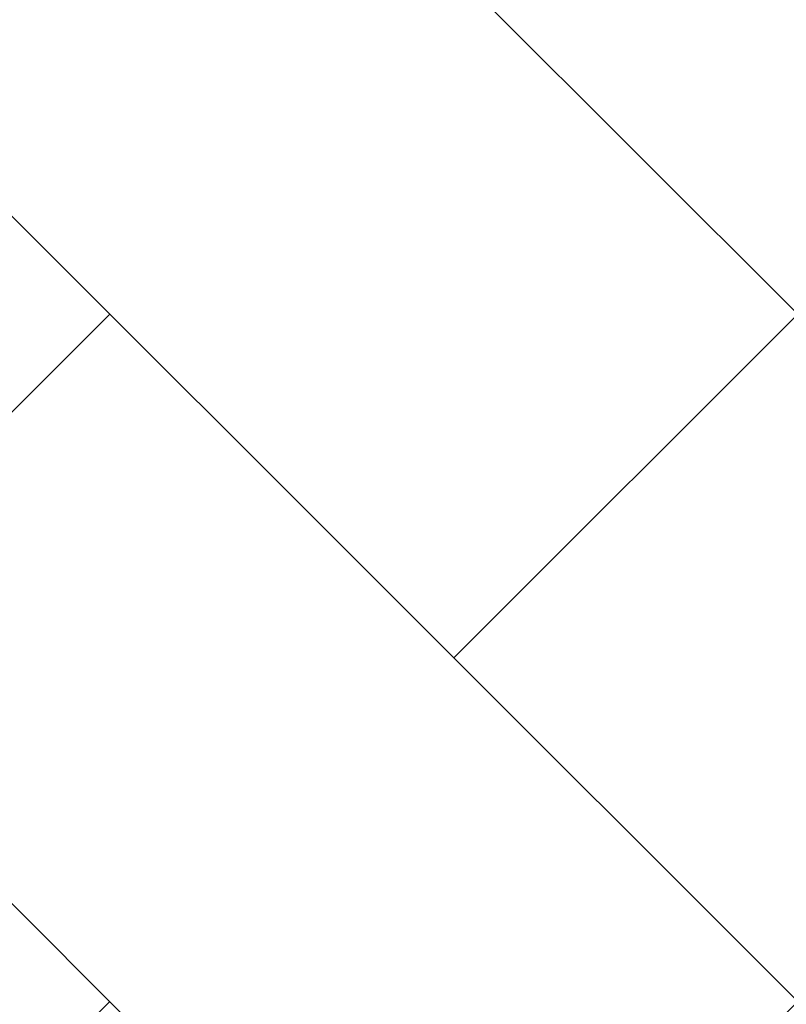
# Model space of a CAD drawing. Units: inches. Extents: x 3590 to 5167, y 65 to 1917.
# Tile 67 of 100: x 4968 to 5000, y 1681 to 1722. Entities that reach past the tile are written whole.
import ezdxf

# ---------------------------------------------------------------- set-up
doc = ezdxf.new("R2010")
doc.units = ezdxf.units.IN
doc.layers.add('A-FLOR-PATT', color=8, linetype='Continuous', lineweight=13)

msp = doc.modelspace()

# ---------------------------------------------------------------- hatches: boundary and pattern name
at = {"layer": 'A-FLOR-PATT', "transparency": 33554687}
h = msp.add_hatch(dxfattribs=at)
h.set_pattern_fill('AR-HBONE', color=256, scale=0.2)
h.set_pattern_definition([(45, (-588.972, 0), (0, 28.73682), [60.96, -20.32]), (135, (-574.604, 14.368), (3e-15, 28.73682), [60.96, -20.32])])
h.paths.add_polyline_path([(5071.274, 1796.999), (4933.274, 1796.999), (4933.274, 1753.999), (4962.774, 1753.999, -0.414214), (4928.774, 1719.999), (4933.274, 1718.999), (4933.274, 1334.999), (5071.274, 1334.999)])
h.paths.add_polyline_path([(4951.78, 1521.077), (4951.715, 1521.04), (4951.563, 1520.895)], flags=16)
h.paths.add_polyline_path([(4952.267, 1521.376), (4952.198, 1521.371), (4952.198, 1521.356)], flags=0)
h.paths.add_polyline_path([(4967.051, 1529.728), (4965.231, 1528.694), (4963.411, 1527.714), (4961.756, 1526.851), (4963.589, 1527.449), (4964.036, 1527.478), (4962.975, 1527.249), (4961.76, 1526.852), (4959.792, 1525.834), (4958.005, 1524.895), (4956.24, 1523.93), (4954.504, 1522.919), (4954.129, 1522.682), (4953.361, 1521.997), (4953.366, 1521.998), (4953.605, 1522.064), (4955.106, 1522.761), (4956.921, 1523.434), (4958.678, 1523.915), (4960.358, 1524.2), (4961.945, 1524.286), (4964.171, 1524.108), (4965.958, 1523.309), (4963.863, 1522.976), (4965.187, 1522.499), (4963.366, 1522.497), (4961.545, 1522.487), (4959.764, 1522.461), (4958.304, 1522.419), (4957.974, 1522.388), (4956.307, 1522.232), (4954.718, 1522.071), (4953.251, 1521.899), (4953.525, 1521.623), (4954.331, 1521.379), (4956.243, 1521.23), (4958.039, 1520.93), (4959.684, 1520.483), (4961.16, 1519.896), (4963.107, 1518.8), (4964.393, 1517.325), (4962.973, 1517.726), (4964.558, 1516.661), (4965.407, 1515.708), (4963.507, 1516.322), (4961.68, 1517.005), (4959.935, 1517.745), (4958.282, 1518.528), (4956.732, 1519.343), (4955.295, 1520.175), (4954.672, 1520.572), (4954.513, 1520.627), (4955.658, 1519.318), (4956.703, 1517.982), (4957.644, 1516.647), (4958.485, 1515.334), (4959.55, 1513.524), (4960.438, 1511.769), (4958.841, 1513.62), (4957.452, 1515.325), (4955.819, 1517.459), (4956.665, 1515.448), (4957.111, 1513.923), (4957.447, 1511.714), (4957.076, 1509.793), (4956.538, 1511.11), (4955.992, 1512.569), (4955.444, 1514.125), (4954.898, 1515.735), (4954.357, 1517.356), (4953.824, 1518.943), (4953.305, 1520.452), (4953.065, 1521.116), (4952.971, 1521.146), (4952.949, 1521.086), (4952.73, 1520.199), (4953.37, 1518.024), (4953.757, 1516.373), (4954.051, 1514.765), (4954.264, 1513.221), (4954.471, 1511.131), (4954.497, 1510.402), (4954.409, 1511.76), (4954.264, 1513.221), (4954.051, 1514.765), (4953.757, 1516.373), (4953.37, 1518.024), (4952.877, 1519.698), (4952.716, 1520.141), (4952.533, 1519.059), (4952.374, 1517.789), (4952.219, 1516.312), (4952.046, 1514.6), (4951.833, 1512.626), (4951.557, 1510.363), (4951.203, 1512.168), (4950.852, 1514.339), (4950.985, 1516.376), (4951.66, 1518.286), (4952.593, 1520.481), (4952.357, 1521.13), (4951.855, 1520.328), (4950.839, 1518.908), (4949.777, 1517.587), (4948.916, 1516.617), (4948.111, 1515.256), (4947.089, 1513.554), (4945.889, 1511.615), (4946.326, 1513.402), (4946.562, 1514.249), (4945.528, 1513.327), (4944.581, 1512.531), (4946.018, 1514.508), (4947.204, 1516.048), (4947.893, 1517.313), (4949.307, 1518.764), (4950.414, 1519.767), (4950.451, 1519.806), (4952.267, 1521.376), (4951.645, 1521.493), (4950.404, 1521.18), (4948.044, 1520.359), (4946.119, 1519.452), (4944.572, 1518.475), (4943.35, 1517.443), (4941.997, 1515.92), (4941.661, 1515.275), (4942.813, 1516.99), (4944.572, 1518.475), (4946.119, 1519.452), (4948.044, 1520.359), (4950.404, 1521.18), (4951.645, 1521.493), (4949.647, 1521.868), (4948.6, 1521.756), (4947.126, 1521.57), (4945.42, 1521.348), (4943.45, 1521.105), (4941.183, 1520.856), (4942.86, 1521.613), (4943.873, 1522.03), (4942.952, 1521.909), (4941.41, 1521.485), (4939.543, 1520.67), (4938.968, 1520.226), (4940.733, 1521.299), (4942.952, 1521.909), (4943.702, 1522.008), (4945.894, 1522.7), (4947.565, 1522.714), (4948.921, 1522.566), (4951.131, 1522.183), (4950.971, 1522.297), (4948.129, 1523.006), (4946.035, 1523.707), (4944.232, 1524.521), (4942.707, 1525.461), (4941.444, 1526.537), (4940.43, 1527.761), (4939.649, 1529.143), (4941.421, 1528.122), (4943.147, 1527.132), (4944.841, 1526.175), (4946.514, 1525.25), (4948.179, 1524.359), (4948.365, 1524.263), (4946.475, 1526.045), (4945.181, 1527.54), (4944.19, 1529.033), (4943.496, 1530.54), (4943.278, 1531.36), (4942.498, 1531.919), (4943.114, 1531.762), (4942.959, 1533.659), (4944.14, 1531.989), (4944.612, 1531.323), (4946.202, 1530.463), (4947.486, 1529.509), (4948.79, 1528.226), (4950.368, 1526.237), (4949.485, 1528.155), (4948.851, 1530.123), (4948.491, 1532.041), (4948.381, 1533.918), (4948.501, 1535.76), (4948.827, 1537.573), (4949.418, 1535.565), (4949.957, 1533.569), (4950.464, 1531.586), (4950.961, 1529.617), (4951.391, 1527.954), (4951.724, 1530.687), (4952.201, 1532.58), (4952.889, 1534.33), (4953.77, 1535.951), (4954.827, 1537.46), (4954.521, 1535.39), (4954.273, 1533.937), (4955.58, 1535.663), (4956.748, 1536.739), (4956.159, 1534.78), (4955.589, 1532.873), (4955.043, 1531.006), (4954.525, 1529.166), (4954.038, 1527.341), (4953.638, 1525.733), (4953.611, 1525.586), (4953.398, 1524.166), (4953.382, 1524.009), (4954.07, 1525.476), (4954.912, 1527.022), (4956.136, 1528.894), (4957.847, 1530.577), (4959.376, 1531.54), (4958.256, 1530.104), (4957.143, 1528.663), (4956.066, 1527.243), (4955.056, 1525.871), (4954.141, 1524.571), (4953.352, 1523.372), (4953.311, 1523.303), (4953.273, 1522.925), (4953.261, 1522.382), (4954.103, 1523.373), (4954.63, 1524.284), (4955.961, 1526.358), (4957.23, 1528.13), (4958.421, 1529.609), (4960.037, 1531.368), (4961.374, 1532.375), (4962.101, 1532.77), (4961.07, 1531.061), (4959.987, 1529.438), (4958.869, 1527.908), (4958.15, 1527.007), (4959.803, 1528.003), (4961.589, 1528.793), (4963.391, 1529.328), (4965.211, 1529.632)], flags=16)
h.paths.add_polyline_path([(4962.944, 1523.182), (4961.107, 1523.422), (4960.392, 1523.362), (4962.35, 1523.331)], flags=0)
h.paths.add_polyline_path([(5049.541, 1584.551), (5049.476, 1584.515), (5049.325, 1584.37)], flags=16)
h.paths.add_polyline_path([(5050.028, 1584.851), (5049.959, 1584.845), (5049.959, 1584.83)], flags=0)
h.paths.add_polyline_path([(5042.333, 1581.949), (5043.88, 1582.926), (5045.806, 1583.833), (5048.165, 1584.654), (5049.406, 1584.967), (5047.408, 1585.342), (5046.361, 1585.231), (5044.888, 1585.044), (5043.181, 1584.822), (5041.211, 1584.579), (5038.944, 1584.33), (5040.622, 1585.087), (5041.634, 1585.504), (5040.713, 1585.383), (5039.171, 1584.959), (5037.304, 1584.144), (5036.729, 1583.7), (5038.494, 1584.773), (5040.713, 1585.383), (5041.463, 1585.482), (5043.655, 1586.174), (5045.326, 1586.188), (5046.682, 1586.04), (5048.893, 1585.657), (5048.732, 1585.771), (5045.891, 1586.48), (5043.796, 1587.181), (5041.994, 1587.996), (5040.468, 1588.935), (5039.205, 1590.011), (5038.191, 1591.235), (5037.41, 1592.617), (5039.182, 1591.596), (5040.909, 1590.607), (5042.602, 1589.649), (5044.275, 1588.724), (5045.94, 1587.833), (5046.126, 1587.738), (5044.237, 1589.519), (5042.942, 1591.015), (5041.952, 1592.508), (5041.257, 1594.014), (5041.039, 1594.834), (5040.26, 1595.393), (5040.875, 1595.237), (5040.721, 1597.133), (5041.901, 1595.463), (5042.373, 1594.798), (5043.963, 1593.938), (5045.247, 1592.983), (5046.552, 1591.701), (5048.129, 1589.712), (5047.247, 1591.63), (5046.613, 1593.597), (5046.252, 1595.515), (5046.142, 1597.392), (5046.262, 1599.234), (5046.588, 1601.047), (5047.179, 1599.039), (5047.718, 1597.043), (5048.225, 1595.06), (5048.722, 1593.091), (5049.152, 1591.429), (5049.485, 1594.161), (5049.962, 1596.054), (5050.65, 1597.804), (5051.532, 1599.425), (5052.589, 1600.934), (5052.283, 1598.864), (5052.034, 1597.411), (5053.341, 1599.137), (5054.509, 1600.213), (5053.92, 1598.254), (5053.35, 1596.348), (5052.805, 1594.48), (5052.286, 1592.64), (5051.799, 1590.815), (5051.4, 1589.207), (5051.373, 1589.06), (5051.159, 1587.64), (5051.143, 1587.483), (5051.831, 1588.95), (5052.673, 1590.496), (5053.898, 1592.368), (5055.608, 1594.051), (5057.137, 1595.014), (5056.017, 1593.578), (5054.904, 1592.137), (5053.828, 1590.717), (5052.817, 1589.345), (5051.902, 1588.046), (5051.113, 1586.846), (5051.072, 1586.777), (5051.034, 1586.399), (5051.022, 1585.856), (5051.864, 1586.847), (5052.391, 1587.758), (5053.723, 1589.832), (5054.991, 1591.604), (5056.182, 1593.083), (5057.798, 1594.842), (5059.135, 1595.849), (5059.863, 1596.244), (5058.831, 1594.535), (5057.749, 1592.912), (5056.63, 1591.382), (5055.912, 1590.482), (5057.564, 1591.477), (5059.35, 1592.267), (5061.152, 1592.802), (5062.972, 1593.106), (5064.812, 1593.203), (5062.992, 1592.169), (5061.172, 1591.188), (5059.518, 1590.325), (5061.35, 1590.924), (5061.797, 1590.952), (5060.737, 1590.723), (5059.521, 1590.326), (5057.553, 1589.308), (5055.766, 1588.369), (5054.002, 1587.404), (5052.265, 1586.393), (5051.891, 1586.156), (5051.122, 1585.471), (5051.127, 1585.472), (5051.366, 1585.538), (5052.867, 1586.235), (5054.682, 1586.908), (5056.439, 1587.389), (5058.12, 1587.675), (5059.706, 1587.76), (5061.933, 1587.583), (5063.719, 1586.783), (5061.624, 1586.45), (5062.949, 1585.973), (5061.127, 1585.971), (5059.307, 1585.961), (5057.525, 1585.935), (5056.065, 1585.893), (5055.735, 1585.862), (5054.068, 1585.707), (5052.479, 1585.546), (5051.012, 1585.373), (5051.286, 1585.097), (5052.092, 1584.853), (5054.004, 1584.704), (5055.8, 1584.404), (5057.446, 1583.958), (5058.921, 1583.37), (5060.868, 1582.274), (5062.154, 1580.799), (5060.734, 1581.2), (5062.32, 1580.135), (5063.168, 1579.182), (5061.269, 1579.796), (5059.441, 1580.479), (5057.696, 1581.219), (5056.043, 1582.003), (5054.493, 1582.817), (5053.057, 1583.649), (5052.433, 1584.047), (5052.274, 1584.101), (5053.42, 1582.793), (5054.464, 1581.457), (5055.405, 1580.121), (5056.247, 1578.809), (5057.311, 1576.998), (5058.199, 1575.244), (5056.602, 1577.094), (5055.213, 1578.799), (5053.58, 1580.933), (5054.427, 1578.922), (5054.872, 1577.397), (5055.208, 1575.189), (5054.838, 1573.267), (5054.299, 1574.584), (5053.754, 1576.043), (5053.206, 1577.599), (5052.659, 1579.209), (5052.118, 1580.83), (5051.585, 1582.417), (5051.066, 1583.927), (5050.826, 1584.59), (5050.733, 1584.62), (5050.711, 1584.561), (5050.491, 1583.673), (5051.131, 1581.498), (5051.518, 1579.847), (5051.813, 1578.24), (5052.026, 1576.695), (5052.233, 1574.605), (5052.258, 1573.876), (5052.17, 1575.234), (5052.026, 1576.695), (5051.813, 1578.24), (5051.518, 1579.847), (5051.131, 1581.498), (5050.638, 1583.172), (5050.477, 1583.615), (5050.294, 1582.533), (5050.136, 1581.263), (5049.981, 1579.786), (5049.807, 1578.074), (5049.594, 1576.1), (5049.318, 1573.837), (5048.965, 1575.642), (5048.613, 1577.813), (5048.747, 1579.85), (5049.421, 1581.76), (5050.354, 1583.955), (5050.118, 1584.604), (5049.616, 1583.802), (5048.6, 1582.382), (5047.538, 1581.061), (5046.677, 1580.091), (5045.872, 1578.73), (5044.85, 1577.028), (5043.651, 1575.089), (5044.087, 1576.877), (5044.324, 1577.723), (5043.289, 1576.801), (5042.342, 1576.005), (5043.779, 1577.982), (5044.966, 1579.522), (5045.655, 1580.787), (5047.068, 1582.239), (5048.175, 1583.241), (5048.213, 1583.28), (5050.028, 1584.851), (5049.406, 1584.967), (5048.165, 1584.654), (5045.806, 1583.833), (5043.88, 1582.926), (5042.333, 1581.949), (5041.111, 1580.917), (5039.758, 1579.394), (5039.423, 1578.749), (5040.575, 1580.464)], flags=16)
h.paths.add_polyline_path([(4954.799, 1533.12), (4954.262, 1532.079), (4953.831, 1530.935), (4953.505, 1529.636), (4953.283, 1528.133), (4953.167, 1526.376), (4953.156, 1524.315), (4953.277, 1521.236), (4952.802, 1521.842), (4951.557, 1521.998), (4950.976, 1521.961), (4952.661, 1521.941), (4952.802, 1521.842), (4953.152, 1523.593), (4953.167, 1526.376), (4953.283, 1528.133), (4953.609, 1530.346), (4954.456, 1532.592)], flags=0)
h.paths.add_polyline_path([(5050.563, 1585.316), (5049.318, 1585.472), (5048.737, 1585.435), (5050.422, 1585.415), (5050.563, 1585.316), (5050.914, 1587.067), (5050.928, 1589.851), (5051.045, 1591.607), (5051.371, 1593.82), (5052.217, 1596.066), (5052.56, 1596.594), (5052.024, 1595.554), (5051.592, 1594.409), (5051.266, 1593.11), (5051.045, 1591.607), (5050.928, 1589.851), (5050.918, 1587.789), (5051.038, 1584.71)], flags=0)
h.paths.add_polyline_path([(5058.153, 1586.836), (5060.111, 1586.805), (5060.705, 1586.656), (5058.868, 1586.896)], flags=0)
h.paths.add_polyline_path([(5049.541, 1430.936), (5049.476, 1430.9), (5049.325, 1430.755)], flags=16)
h.paths.add_polyline_path([(5050.028, 1431.236), (5049.959, 1431.231), (5049.959, 1431.215)], flags=0)
h.paths.add_polyline_path([(5046.588, 1447.432), (5047.179, 1445.425), (5047.718, 1443.429), (5048.225, 1441.446), (5048.722, 1439.476), (5049.152, 1437.814), (5049.485, 1440.546), (5049.962, 1442.439), (5050.65, 1444.189), (5051.532, 1445.811), (5052.589, 1447.319), (5052.283, 1445.249), (5052.034, 1443.796), (5053.341, 1445.522), (5054.509, 1446.598), (5053.92, 1444.64), (5053.35, 1442.733), (5052.805, 1440.865), (5052.286, 1439.025), (5051.799, 1437.201), (5051.4, 1435.592), (5051.373, 1435.445), (5051.159, 1434.025), (5051.143, 1433.868), (5051.831, 1435.335), (5052.673, 1436.881), (5053.898, 1438.753), (5055.608, 1440.436), (5057.137, 1441.4), (5056.017, 1439.963), (5054.904, 1438.522), (5053.828, 1437.102), (5052.817, 1435.73), (5051.902, 1434.431), (5051.113, 1433.231), (5051.072, 1433.162), (5051.034, 1432.784), (5051.022, 1432.242), (5051.864, 1433.232), (5052.391, 1434.143), (5053.723, 1436.217), (5054.991, 1437.989), (5056.182, 1439.468), (5057.798, 1441.227), (5059.135, 1442.235), (5059.863, 1442.629), (5058.831, 1440.921), (5057.749, 1439.298), (5056.63, 1437.767), (5055.912, 1436.867), (5057.564, 1437.863), (5059.35, 1438.652), (5061.152, 1439.187), (5062.972, 1439.491), (5064.812, 1439.588), (5062.992, 1438.554), (5061.172, 1437.573), (5059.518, 1436.71), (5061.35, 1437.309), (5061.797, 1437.337), (5060.737, 1437.108), (5059.521, 1436.711), (5057.553, 1435.693), (5055.766, 1434.754), (5054.002, 1433.789), (5052.265, 1432.778), (5051.891, 1432.541), (5051.122, 1431.856), (5051.127, 1431.857), (5051.366, 1431.923), (5052.867, 1432.62), (5054.682, 1433.293), (5056.439, 1433.775), (5058.12, 1434.06), (5059.706, 1434.145), (5061.933, 1433.968), (5063.719, 1433.168), (5061.624, 1432.835), (5062.949, 1432.358), (5061.127, 1432.357), (5059.307, 1432.346), (5057.525, 1432.32), (5056.065, 1432.278), (5055.735, 1432.248), (5054.068, 1432.092), (5052.479, 1431.931), (5051.012, 1431.759), (5051.286, 1431.482), (5052.092, 1431.238), (5054.004, 1431.089), (5055.8, 1430.789), (5057.446, 1430.343), (5058.921, 1429.755), (5060.868, 1428.66), (5062.154, 1427.185), (5060.734, 1427.585), (5062.32, 1426.52), (5063.168, 1425.567), (5061.269, 1426.181), (5059.441, 1426.865), (5057.696, 1427.604), (5056.043, 1428.388), (5054.493, 1429.202), (5053.057, 1430.034), (5052.433, 1430.432), (5052.274, 1430.487), (5053.42, 1429.178), (5054.464, 1427.842), (5055.405, 1426.506), (5056.247, 1425.194), (5057.311, 1423.383), (5058.199, 1421.629), (5056.602, 1423.479), (5055.213, 1425.184), (5053.58, 1427.318), (5054.427, 1425.307), (5054.872, 1423.782), (5055.208, 1421.574), (5054.838, 1419.652), (5054.299, 1420.97), (5053.754, 1422.428), (5053.206, 1423.984), (5052.659, 1425.595), (5052.118, 1427.215), (5051.585, 1428.802), (5051.066, 1430.312), (5050.826, 1430.975), (5050.733, 1431.005), (5050.711, 1430.946), (5050.491, 1430.058), (5051.131, 1427.883), (5051.518, 1426.232), (5051.813, 1424.625), (5052.026, 1423.081), (5052.233, 1420.991), (5052.258, 1420.261), (5052.17, 1421.619), (5052.026, 1423.081), (5051.813, 1424.625), (5051.518, 1426.232), (5051.131, 1427.883), (5050.638, 1429.558), (5050.477, 1430.001), (5050.294, 1428.918), (5050.136, 1427.648), (5049.981, 1426.171), (5049.807, 1424.459), (5049.594, 1422.485), (5049.318, 1420.222), (5048.965, 1422.028), (5048.613, 1424.199), (5048.747, 1426.235), (5049.421, 1428.146), (5050.354, 1430.34), (5050.118, 1430.989), (5049.616, 1430.187), (5048.6, 1428.768), (5047.538, 1427.446), (5046.677, 1426.477), (5045.872, 1425.116), (5044.85, 1423.413), (5043.651, 1421.474), (5044.087, 1423.262), (5044.324, 1424.109), (5043.289, 1423.186), (5042.342, 1422.391), (5043.779, 1424.368), (5044.966, 1425.907), (5045.655, 1427.173), (5047.068, 1428.624), (5048.175, 1429.627), (5048.213, 1429.666), (5050.028, 1431.236), (5049.406, 1431.353), (5048.165, 1431.039), (5045.806, 1430.218), (5043.88, 1429.311), (5042.333, 1428.334), (5041.111, 1427.302), (5039.758, 1425.779), (5039.423, 1425.134), (5040.575, 1426.849), (5042.333, 1428.334), (5043.88, 1429.311), (5045.806, 1430.218), (5048.165, 1431.039), (5049.406, 1431.353), (5047.408, 1431.727), (5046.361, 1431.616), (5044.888, 1431.429), (5043.181, 1431.207), (5041.211, 1430.964), (5038.944, 1430.715), (5040.622, 1431.472), (5041.634, 1431.89), (5040.713, 1431.769), (5039.171, 1431.345), (5037.304, 1430.53), (5036.729, 1430.085), (5038.494, 1431.158), (5040.713, 1431.769), (5041.463, 1431.867), (5043.655, 1432.559), (5045.326, 1432.573), (5046.682, 1432.425), (5048.893, 1432.042), (5048.732, 1432.156), (5045.891, 1432.865), (5043.796, 1433.566), (5041.994, 1434.381), (5040.468, 1435.321), (5039.205, 1436.396), (5038.191, 1437.62), (5037.41, 1439.002), (5039.182, 1437.982), (5040.909, 1436.992), (5042.602, 1436.034), (5044.275, 1435.109), (5045.94, 1434.218), (5046.126, 1434.123), (5044.237, 1435.904), (5042.942, 1437.4), (5041.952, 1438.893), (5041.257, 1440.399), (5041.039, 1441.219), (5040.26, 1441.778), (5040.875, 1441.622), (5040.721, 1443.518), (5041.901, 1441.848), (5042.373, 1441.183), (5043.963, 1440.323), (5045.247, 1439.369), (5046.552, 1438.086), (5048.129, 1436.097), (5047.247, 1438.015), (5046.613, 1439.982), (5046.252, 1441.901), (5046.142, 1443.778), (5046.262, 1445.619)], flags=16)
h.paths.add_polyline_path([(5052.382, 1444.255), (5051.623, 1442.78), (5052.024, 1441.939), (5052.56, 1442.98)], flags=0)
h.paths.add_polyline_path([(5050.563, 1431.701), (5049.318, 1431.857), (5048.737, 1431.821), (5050.422, 1431.8)], flags=0)
h.paths.add_polyline_path([(5058.153, 1433.221), (5060.111, 1433.19), (5060.705, 1433.041), (5058.868, 1433.281)], flags=0)
h.paths.add_polyline_path([(5049.541, 1352.285), (5049.476, 1352.249), (5049.325, 1352.104)], flags=16)
h.paths.add_polyline_path([(5050.028, 1352.585), (5049.959, 1352.58), (5049.959, 1352.564)], flags=0)
h.paths.add_polyline_path([(5046.588, 1368.781), (5047.179, 1366.774), (5047.718, 1364.778), (5048.225, 1362.795), (5048.722, 1360.825), (5049.152, 1359.163), (5049.485, 1361.896), (5049.962, 1363.789), (5050.65, 1365.538), (5051.532, 1367.16), (5052.589, 1368.669), (5052.283, 1366.598), (5052.034, 1365.145), (5053.341, 1366.871), (5054.509, 1367.947), (5053.92, 1365.989), (5053.35, 1364.082), (5052.805, 1362.214), (5052.286, 1360.374), (5051.799, 1358.55), (5051.4, 1356.942), (5051.373, 1356.794), (5051.159, 1355.374), (5051.143, 1355.218), (5051.831, 1356.684), (5052.673, 1358.23), (5053.898, 1360.102), (5055.608, 1361.786), (5057.137, 1362.749), (5056.017, 1361.313), (5054.904, 1359.872), (5053.828, 1358.452), (5052.817, 1357.079), (5051.902, 1355.78), (5051.113, 1354.581), (5051.072, 1354.512), (5051.034, 1354.133), (5051.022, 1353.591), (5051.864, 1354.581), (5052.391, 1355.492), (5053.723, 1357.566), (5054.991, 1359.338), (5056.182, 1360.817), (5057.798, 1362.577), (5059.135, 1363.584), (5059.863, 1363.979), (5058.831, 1362.27), (5057.749, 1360.647), (5056.63, 1359.117), (5055.912, 1358.216), (5057.564, 1359.212), (5059.35, 1360.001), (5061.152, 1360.536), (5062.972, 1360.841), (5064.812, 1360.937), (5062.992, 1359.903), (5061.172, 1358.923), (5059.518, 1358.059), (5061.35, 1358.658), (5061.797, 1358.687), (5060.737, 1358.458), (5059.521, 1358.061), (5057.553, 1357.043), (5055.766, 1356.103), (5054.002, 1355.138), (5052.265, 1354.127), (5051.891, 1353.89), (5051.122, 1353.206), (5051.127, 1353.206), (5051.366, 1353.272), (5052.867, 1353.969), (5054.682, 1354.643), (5056.439, 1355.124), (5058.12, 1355.409), (5059.706, 1355.495), (5061.933, 1355.317), (5063.719, 1354.518), (5061.624, 1354.184), (5062.949, 1353.708), (5061.127, 1353.706), (5059.307, 1353.695), (5057.525, 1353.669), (5056.065, 1353.627), (5055.735, 1353.597), (5054.068, 1353.441), (5052.479, 1353.28), (5051.012, 1353.108), (5051.286, 1352.831), (5052.092, 1352.587), (5054.004, 1352.439), (5055.8, 1352.138), (5057.446, 1351.692), (5058.921, 1351.104), (5060.868, 1350.009), (5062.154, 1348.534), (5060.734, 1348.935), (5062.32, 1347.869), (5063.168, 1346.916), (5061.269, 1347.53), (5059.441, 1348.214), (5057.696, 1348.954), (5056.043, 1349.737), (5054.493, 1350.551), (5053.057, 1351.383), (5052.433, 1351.781), (5052.274, 1351.836), (5053.42, 1350.527), (5054.464, 1349.191), (5055.405, 1347.855), (5056.247, 1346.543), (5057.311, 1344.733), (5058.199, 1342.978), (5056.602, 1344.828), (5055.213, 1346.534), (5053.58, 1348.667), (5054.427, 1346.656), (5054.872, 1345.132), (5055.208, 1342.923), (5054.838, 1341.002), (5054.299, 1342.319), (5053.754, 1343.778), (5053.206, 1345.334), (5052.659, 1346.944), (5052.118, 1348.564), (5051.585, 1350.151), (5051.066, 1351.661), (5050.826, 1352.324), (5050.733, 1352.355), (5050.711, 1352.295), (5050.491, 1351.408), (5051.131, 1349.232), (5051.518, 1347.581), (5051.813, 1345.974), (5052.026, 1344.43), (5052.233, 1342.34), (5052.258, 1341.61), (5052.17, 1342.969), (5052.026, 1344.43), (5051.813, 1345.974), (5051.518, 1347.581), (5051.131, 1349.232), (5050.638, 1350.907), (5050.477, 1351.35), (5050.294, 1350.267), (5050.136, 1348.997), (5049.981, 1347.52), (5049.807, 1345.809), (5049.594, 1343.835), (5049.318, 1341.571), (5048.965, 1343.377), (5048.613, 1345.548), (5048.747, 1347.585), (5049.421, 1349.495), (5050.354, 1351.689), (5050.118, 1352.339), (5049.616, 1351.536), (5048.6, 1350.117), (5047.538, 1348.795), (5046.677, 1347.826), (5045.872, 1346.465), (5044.85, 1344.763), (5043.651, 1342.824), (5044.087, 1344.611), (5044.324, 1345.458), (5043.289, 1344.535), (5042.342, 1343.74), (5043.779, 1345.717), (5044.966, 1347.256), (5045.655, 1348.522), (5047.068, 1349.973), (5048.175, 1350.976), (5048.213, 1351.015), (5050.028, 1352.585), (5049.406, 1352.702), (5048.165, 1352.388), (5045.806, 1351.567), (5043.88, 1350.661), (5042.333, 1349.683), (5041.111, 1348.651), (5039.758, 1347.128), (5039.423, 1346.483), (5040.575, 1348.198), (5042.333, 1349.683), (5043.88, 1350.661), (5045.806, 1351.567), (5048.165, 1352.388), (5049.406, 1352.702), (5047.408, 1353.076), (5046.361, 1352.965), (5044.888, 1352.779), (5043.181, 1352.556), (5041.211, 1352.313), (5038.944, 1352.065), (5040.622, 1352.821), (5041.634, 1353.239), (5040.713, 1353.118), (5039.171, 1352.694), (5037.304, 1351.879), (5036.729, 1351.434), (5038.494, 1352.508), (5040.713, 1353.118), (5041.463, 1353.216), (5043.655, 1353.909), (5045.326, 1353.923), (5046.682, 1353.774), (5048.893, 1353.391), (5048.732, 1353.506), (5045.891, 1354.214), (5043.796, 1354.915), (5041.994, 1355.73), (5040.468, 1356.67), (5039.205, 1357.746), (5038.191, 1358.969), (5037.41, 1360.352), (5039.182, 1359.331), (5040.909, 1358.341), (5042.602, 1357.383), (5044.275, 1356.458), (5045.94, 1355.567), (5046.126, 1355.472), (5044.237, 1357.253), (5042.942, 1358.749), (5041.952, 1360.242), (5041.257, 1361.748), (5041.039, 1362.568), (5040.26, 1363.128), (5040.875, 1362.971), (5040.721, 1364.867), (5041.901, 1363.197), (5042.373, 1362.532), (5043.963, 1361.672), (5045.247, 1360.718), (5046.552, 1359.435), (5048.129, 1357.446), (5047.247, 1359.364), (5046.613, 1361.331), (5046.252, 1363.25), (5046.142, 1365.127), (5046.262, 1366.969)], flags=16)
h.paths.add_polyline_path([(5052.382, 1365.604), (5051.623, 1364.129), (5052.024, 1363.288), (5052.56, 1364.329)], flags=0)
h.paths.add_polyline_path([(4951.78, 1698.041), (4951.715, 1698.005), (4951.563, 1697.859)], flags=16)
h.paths.add_polyline_path([(4952.267, 1698.341), (4952.198, 1698.335), (4952.198, 1698.32)], flags=0)
h.paths.add_polyline_path([(4957.076, 1686.757), (4956.538, 1688.074), (4955.992, 1689.533), (4955.444, 1691.089), (4954.898, 1692.699), (4954.357, 1694.32), (4953.824, 1695.907), (4953.305, 1697.417), (4953.065, 1698.08), (4952.971, 1698.11), (4952.949, 1698.051), (4952.73, 1697.163), (4953.37, 1694.988), (4953.757, 1693.337), (4954.051, 1691.729), (4954.264, 1690.185), (4954.471, 1688.095), (4954.497, 1687.366), (4954.409, 1688.724), (4954.264, 1690.185), (4954.051, 1691.729), (4953.757, 1693.337), (4953.37, 1694.988), (4952.877, 1696.662), (4952.716, 1697.105), (4952.533, 1696.023), (4952.374, 1694.753), (4952.219, 1693.276), (4952.046, 1691.564), (4951.833, 1689.59), (4951.557, 1687.327), (4951.203, 1689.132), (4950.852, 1691.303), (4950.985, 1693.34), (4951.66, 1695.25), (4952.593, 1697.445), (4952.357, 1698.094), (4951.855, 1697.292), (4950.839, 1695.872), (4949.777, 1694.551), (4948.916, 1693.581), (4948.111, 1692.22), (4947.089, 1690.518), (4945.889, 1688.579), (4946.326, 1690.366), (4946.562, 1691.213), (4945.528, 1690.291), (4944.581, 1689.495), (4946.018, 1691.472), (4947.204, 1693.012), (4947.893, 1694.277), (4949.307, 1695.729), (4950.414, 1696.731), (4950.451, 1696.77), (4952.267, 1698.341), (4951.645, 1698.457), (4950.404, 1698.144), (4948.044, 1697.323), (4946.119, 1696.416), (4944.572, 1695.439), (4943.35, 1694.407), (4941.997, 1692.884), (4941.661, 1692.239), (4942.813, 1693.954), (4944.572, 1695.439), (4946.119, 1696.416), (4948.044, 1697.323), (4950.404, 1698.144), (4951.645, 1698.457), (4949.647, 1698.832), (4948.6, 1698.72), (4947.126, 1698.534), (4945.42, 1698.312), (4943.45, 1698.069), (4941.183, 1697.82), (4942.86, 1698.577), (4943.873, 1698.994), (4942.952, 1698.873), (4941.41, 1698.449), (4939.543, 1697.634), (4938.968, 1697.19), (4940.733, 1698.263), (4942.952, 1698.873), (4943.702, 1698.972), (4945.894, 1699.664), (4947.565, 1699.678), (4948.921, 1699.53), (4951.131, 1699.147), (4950.971, 1699.261), (4948.129, 1699.97), (4946.035, 1700.671), (4944.232, 1701.486), (4942.707, 1702.425), (4941.444, 1703.501), (4940.43, 1704.725), (4939.649, 1706.107), (4941.421, 1705.086), (4943.147, 1704.097), (4944.841, 1703.139), (4946.514, 1702.214), (4948.179, 1701.323), (4948.365, 1701.227), (4946.475, 1703.009), (4945.181, 1704.505), (4944.19, 1705.997), (4943.496, 1707.504), (4943.278, 1708.324), (4942.498, 1708.883), (4943.114, 1708.727), (4942.959, 1710.623), (4944.14, 1708.953), (4944.612, 1708.287), (4946.202, 1707.428), (4947.486, 1706.473), (4948.79, 1705.191), (4950.368, 1703.202), (4949.485, 1705.12), (4948.851, 1707.087), (4948.491, 1709.005), (4948.381, 1710.882), (4948.501, 1712.724), (4948.827, 1714.537), (4949.418, 1712.529), (4949.957, 1710.533), (4950.464, 1708.55), (4950.961, 1706.581), (4951.391, 1704.919), (4951.724, 1707.651), (4952.201, 1709.544), (4952.889, 1711.294), (4953.77, 1712.915), (4954.827, 1714.424), (4954.521, 1712.354), (4954.273, 1710.901), (4955.58, 1712.627), (4956.748, 1713.703), (4956.159, 1711.744), (4955.589, 1709.837), (4955.043, 1707.97), (4954.525, 1706.13), (4954.038, 1704.305), (4953.638, 1702.697), (4953.611, 1702.55), (4953.398, 1701.13), (4953.382, 1700.973), (4954.07, 1702.44), (4954.912, 1703.986), (4956.136, 1705.858), (4957.847, 1707.541), (4959.376, 1708.504), (4958.256, 1707.068), (4957.143, 1705.627), (4956.066, 1704.207), (4955.056, 1702.835), (4954.141, 1701.536), (4953.352, 1700.336), (4953.311, 1700.267), (4953.273, 1699.889), (4953.261, 1699.346), (4954.103, 1700.337), (4954.63, 1701.248), (4955.961, 1703.322), (4957.23, 1705.094), (4958.421, 1706.573), (4960.037, 1708.332), (4961.374, 1709.339), (4962.101, 1709.734), (4961.07, 1708.025), (4959.987, 1706.402), (4958.869, 1704.872), (4958.15, 1703.972), (4959.803, 1704.967), (4961.589, 1705.757), (4963.391, 1706.292), (4965.211, 1706.596), (4967.051, 1706.692), (4965.231, 1705.659), (4963.411, 1704.678), (4961.756, 1703.815), (4963.589, 1704.413), (4964.036, 1704.442), (4962.975, 1704.213), (4961.76, 1703.816), (4959.792, 1702.798), (4958.005, 1701.859), (4956.24, 1700.894), (4954.504, 1699.883), (4954.129, 1699.646), (4953.361, 1698.961), (4953.366, 1698.962), (4953.605, 1699.028), (4955.106, 1699.725), (4956.921, 1700.398), (4958.678, 1700.879), (4960.358, 1701.164), (4961.945, 1701.25), (4964.171, 1701.073), (4965.958, 1700.273), (4963.863, 1699.94), (4965.187, 1699.463), (4963.366, 1699.461), (4961.545, 1699.451), (4959.764, 1699.425), (4958.304, 1699.383), (4957.974, 1699.352), (4956.307, 1699.197), (4954.718, 1699.036), (4953.251, 1698.863), (4953.525, 1698.587), (4954.331, 1698.343), (4956.243, 1698.194), (4958.039, 1697.894), (4959.684, 1697.447), (4961.16, 1696.86), (4963.107, 1695.764), (4964.393, 1694.289), (4962.973, 1694.69), (4964.558, 1693.625), (4965.407, 1692.672), (4963.507, 1693.286), (4961.68, 1693.969), (4959.935, 1694.709), (4958.282, 1695.492), (4956.732, 1696.307), (4955.295, 1697.139), (4954.672, 1697.536), (4954.513, 1697.591), (4955.658, 1696.282), (4956.703, 1694.946), (4957.644, 1693.611), (4958.485, 1692.298), (4959.55, 1690.488), (4960.438, 1688.733), (4958.841, 1690.584), (4957.452, 1692.289), (4955.819, 1694.423), (4956.665, 1692.412), (4957.111, 1690.887), (4957.447, 1688.678)], flags=16)
h.paths.add_polyline_path([(5050.563, 1353.05), (5049.318, 1353.207), (5048.737, 1353.17), (5050.422, 1353.15)], flags=0)
h.paths.add_polyline_path([(4951.78, 1351.486), (4951.715, 1351.45), (4951.563, 1351.305)], flags=16)
h.paths.add_polyline_path([(4952.267, 1351.786), (4952.198, 1351.78), (4952.198, 1351.765)], flags=0)
h.paths.add_polyline_path([(4954.827, 1367.869), (4954.521, 1365.799), (4954.273, 1364.346), (4955.58, 1366.072), (4956.748, 1367.148), (4956.159, 1365.19), (4955.589, 1363.283), (4955.043, 1361.415), (4954.525, 1359.575), (4954.038, 1357.751), (4953.638, 1356.142), (4953.611, 1355.995), (4953.398, 1354.575), (4953.382, 1354.418), (4954.07, 1355.885), (4954.912, 1357.431), (4956.136, 1359.303), (4957.847, 1360.986), (4959.376, 1361.95), (4958.256, 1360.513), (4957.143, 1359.072), (4956.066, 1357.652), (4955.056, 1356.28), (4954.141, 1354.981), (4953.352, 1353.781), (4953.311, 1353.712), (4953.273, 1353.334), (4953.261, 1352.792), (4954.103, 1353.782), (4954.63, 1354.693), (4955.961, 1356.767), (4957.23, 1358.539), (4958.421, 1360.018), (4960.037, 1361.777), (4961.374, 1362.785), (4962.101, 1363.179), (4961.07, 1361.471), (4959.987, 1359.848), (4958.869, 1358.317), (4958.15, 1357.417), (4959.803, 1358.413), (4961.589, 1359.202), (4963.391, 1359.737), (4965.211, 1360.041), (4967.051, 1360.138), (4965.231, 1359.104), (4963.411, 1358.123), (4961.756, 1357.26), (4963.589, 1357.859), (4964.036, 1357.887), (4962.975, 1357.658), (4961.76, 1357.261), (4959.792, 1356.243), (4958.005, 1355.304), (4956.24, 1354.339), (4954.504, 1353.328), (4954.129, 1353.091), (4953.361, 1352.406), (4953.366, 1352.407), (4953.605, 1352.473), (4955.106, 1353.17), (4956.921, 1353.843), (4958.678, 1354.325), (4960.358, 1354.61), (4961.945, 1354.695), (4964.171, 1354.518), (4965.958, 1353.718), (4963.863, 1353.385), (4965.187, 1352.908), (4963.366, 1352.907), (4961.545, 1352.896), (4959.764, 1352.87), (4958.304, 1352.828), (4957.974, 1352.798), (4956.307, 1352.642), (4954.718, 1352.481), (4953.251, 1352.309), (4953.525, 1352.032), (4954.331, 1351.788), (4956.243, 1351.639), (4958.039, 1351.339), (4959.684, 1350.893), (4961.16, 1350.305), (4963.107, 1349.21), (4964.393, 1347.735), (4962.973, 1348.135), (4964.558, 1347.07), (4965.407, 1346.117), (4963.507, 1346.731), (4961.68, 1347.414), (4959.935, 1348.154), (4958.282, 1348.938), (4956.732, 1349.752), (4955.295, 1350.584), (4954.672, 1350.982), (4954.513, 1351.036), (4955.658, 1349.728), (4956.703, 1348.392), (4957.644, 1347.056), (4958.485, 1345.744), (4959.55, 1343.933), (4960.438, 1342.179), (4958.841, 1344.029), (4957.452, 1345.734), (4955.819, 1347.868), (4956.665, 1345.857), (4957.111, 1344.332), (4957.447, 1342.124), (4957.076, 1340.202), (4956.538, 1341.52), (4955.992, 1342.978), (4955.444, 1344.534), (4954.898, 1346.145), (4954.357, 1347.765), (4953.824, 1349.352), (4953.305, 1350.862), (4953.065, 1351.525), (4952.971, 1351.555), (4952.949, 1351.496), (4952.73, 1350.608), (4953.37, 1348.433), (4953.757, 1346.782), (4954.051, 1345.175), (4954.264, 1343.631), (4954.471, 1341.541), (4954.497, 1340.811), (4954.409, 1342.169), (4954.264, 1343.631), (4954.051, 1345.175), (4953.757, 1346.782), (4953.37, 1348.433), (4952.877, 1350.108), (4952.716, 1350.551), (4952.533, 1349.468), (4952.374, 1348.198), (4952.219, 1346.721), (4952.046, 1345.009), (4951.833, 1343.035), (4951.557, 1340.772), (4951.203, 1342.578), (4950.852, 1344.749), (4950.985, 1346.785), (4951.66, 1348.696), (4952.593, 1350.89), (4952.357, 1351.539), (4951.855, 1350.737), (4950.839, 1349.318), (4949.777, 1347.996), (4948.916, 1347.027), (4948.111, 1345.665), (4947.089, 1343.963), (4945.889, 1342.024), (4946.326, 1343.812), (4946.562, 1344.659), (4945.528, 1343.736), (4944.581, 1342.941), (4946.018, 1344.918), (4947.204, 1346.457), (4947.893, 1347.723), (4949.307, 1349.174), (4950.414, 1350.177), (4950.451, 1350.216), (4952.267, 1351.786), (4951.645, 1351.903), (4950.404, 1351.589), (4948.044, 1350.768), (4946.119, 1349.861), (4944.572, 1348.884), (4943.35, 1347.852), (4941.997, 1346.329), (4941.661, 1345.684), (4942.813, 1347.399), (4944.572, 1348.884), (4946.119, 1349.861), (4948.044, 1350.768), (4950.404, 1351.589), (4951.645, 1351.903), (4949.647, 1352.277), (4948.6, 1352.166), (4947.126, 1351.979), (4945.42, 1351.757), (4943.45, 1351.514), (4941.183, 1351.265), (4942.86, 1352.022), (4943.873, 1352.44), (4942.952, 1352.319), (4941.41, 1351.895), (4939.543, 1351.08), (4938.968, 1350.635), (4940.733, 1351.708), (4942.952, 1352.319), (4943.702, 1352.417), (4945.894, 1353.109), (4947.565, 1353.123), (4948.921, 1352.975), (4951.131, 1352.592), (4950.971, 1352.706), (4948.129, 1353.415), (4946.035, 1354.116), (4944.232, 1354.931), (4942.707, 1355.871), (4941.444, 1356.946), (4940.43, 1358.17), (4939.649, 1359.552), (4941.421, 1358.532), (4943.147, 1357.542), (4944.841, 1356.584), (4946.514, 1355.659), (4948.179, 1354.768), (4948.365, 1354.673), (4946.475, 1356.454), (4945.181, 1357.95), (4944.19, 1359.443), (4943.496, 1360.949), (4943.278, 1361.769), (4942.498, 1362.328), (4943.114, 1362.172), (4942.959, 1364.068), (4944.14, 1362.398), (4944.612, 1361.733), (4946.202, 1360.873), (4947.486, 1359.919), (4948.79, 1358.636), (4950.368, 1356.647), (4949.485, 1358.565), (4948.851, 1360.532), (4948.491, 1362.451), (4948.381, 1364.328), (4948.501, 1366.169), (4948.827, 1367.982), (4949.418, 1365.975), (4949.957, 1363.979), (4950.464, 1361.995), (4950.961, 1360.026), (4951.391, 1358.364), (4951.724, 1361.096), (4952.201, 1362.989), (4952.889, 1364.739), (4953.77, 1366.361)], flags=16)
h.paths.add_polyline_path([(4954.799, 1363.53), (4954.262, 1362.489), (4953.831, 1361.344), (4953.505, 1360.045), (4953.283, 1358.543), (4953.167, 1356.786), (4953.156, 1354.724), (4953.277, 1351.646), (4952.802, 1352.251), (4951.557, 1352.407), (4950.976, 1352.371), (4952.661, 1352.35), (4952.802, 1352.251), (4953.152, 1354.002), (4953.167, 1356.786), (4953.283, 1358.543), (4953.609, 1360.755), (4954.456, 1363.001)], flags=0)
h.paths.add_polyline_path([(4952.802, 1698.806), (4951.557, 1698.962), (4950.976, 1698.925), (4952.661, 1698.905), (4952.802, 1698.806), (4953.152, 1700.557), (4953.167, 1703.34), (4953.283, 1705.097), (4953.609, 1707.31), (4954.456, 1709.556), (4954.799, 1710.084), (4954.262, 1709.043), (4953.831, 1707.899), (4953.505, 1706.6), (4953.283, 1705.097), (4953.167, 1703.34), (4953.156, 1701.279), (4953.277, 1698.2)], flags=0)
h.paths.add_polyline_path([(4962.944, 1700.146), (4961.107, 1700.386), (4960.392, 1700.326), (4962.35, 1700.295)], flags=0)
h.paths.add_polyline_path([(5058.153, 1354.57), (5060.111, 1354.539), (5060.705, 1354.391), (5058.868, 1354.631)], flags=0)
h.paths.add_polyline_path([(4962.944, 1353.591), (4961.107, 1353.831), (4960.392, 1353.771), (4962.35, 1353.74)], flags=0)
h.paths.add_polyline_path([(5049.541, 1778.72), (5049.476, 1778.684), (5049.325, 1778.539)], flags=16)
h.paths.add_polyline_path([(5050.028, 1779.02), (5049.959, 1779.014), (5049.959, 1778.999)], flags=0)
h.paths.add_polyline_path([(5052.258, 1768.045), (5052.17, 1769.403), (5052.026, 1770.864), (5051.813, 1772.409), (5051.518, 1774.016), (5051.131, 1775.667), (5050.638, 1777.341), (5050.477, 1777.784), (5050.294, 1776.702), (5050.136, 1775.432), (5049.981, 1773.955), (5049.807, 1772.243), (5049.594, 1770.269), (5049.318, 1768.006), (5048.965, 1769.811), (5048.613, 1771.982), (5048.747, 1774.019), (5049.421, 1775.929), (5050.354, 1778.124), (5050.118, 1778.773), (5049.616, 1777.971), (5048.6, 1776.551), (5047.538, 1775.23), (5046.677, 1774.26), (5045.872, 1772.899), (5044.85, 1771.197), (5043.651, 1769.258), (5044.087, 1771.046), (5044.324, 1771.892), (5043.289, 1770.97), (5042.342, 1770.174), (5043.779, 1772.151), (5044.966, 1773.691), (5045.655, 1774.956), (5047.068, 1776.408), (5048.175, 1777.41), (5048.213, 1777.449), (5050.028, 1779.02), (5049.406, 1779.136), (5048.165, 1778.823), (5045.806, 1778.002), (5043.88, 1777.095), (5042.333, 1776.118), (5041.111, 1775.086), (5039.758, 1773.563), (5039.423, 1772.918), (5040.575, 1774.633), (5042.333, 1776.118), (5043.88, 1777.095), (5045.806, 1778.002), (5048.165, 1778.823), (5049.406, 1779.136), (5047.408, 1779.511), (5046.361, 1779.4), (5044.888, 1779.213), (5043.181, 1778.991), (5041.211, 1778.748), (5038.944, 1778.499), (5040.622, 1779.256), (5041.634, 1779.673), (5040.713, 1779.552), (5039.171, 1779.128), (5037.304, 1778.313), (5036.729, 1777.869), (5038.494, 1778.942), (5040.713, 1779.552), (5041.463, 1779.651), (5043.655, 1780.343), (5045.326, 1780.357), (5046.682, 1780.209), (5048.893, 1779.826), (5048.732, 1779.94), (5045.891, 1780.649), (5043.796, 1781.35), (5041.994, 1782.165), (5040.468, 1783.104), (5039.205, 1784.18), (5038.191, 1785.404), (5037.41, 1786.786), (5039.182, 1785.765), (5040.909, 1784.776), (5042.602, 1783.818), (5044.275, 1782.893), (5045.94, 1782.002), (5046.126, 1781.907), (5044.237, 1783.688), (5042.942, 1785.184), (5041.952, 1786.677), (5041.257, 1788.183), (5041.039, 1789.003), (5040.26, 1789.562), (5040.875, 1789.406), (5040.721, 1791.302), (5041.901, 1789.632), (5042.373, 1788.967), (5043.963, 1788.107), (5045.247, 1787.152), (5046.552, 1785.87), (5048.129, 1783.881), (5047.247, 1785.799), (5046.613, 1787.766), (5046.252, 1789.684), (5046.142, 1791.561), (5046.262, 1793.403), (5046.588, 1795.216), (5047.179, 1793.208), (5047.718, 1791.213), (5048.225, 1789.229), (5048.722, 1787.26), (5049.152, 1785.598), (5049.485, 1788.33), (5049.962, 1790.223), (5050.65, 1791.973), (5051.532, 1793.594), (5052.589, 1795.103), (5052.283, 1793.033), (5052.034, 1791.58), (5053.341, 1793.306), (5054.509, 1794.382), (5053.92, 1792.423), (5053.35, 1790.517), (5052.805, 1788.649), (5052.286, 1786.809), (5051.799, 1784.984), (5051.4, 1783.376), (5051.373, 1783.229), (5051.159, 1781.809), (5051.143, 1781.652), (5051.831, 1783.119), (5052.673, 1784.665), (5053.898, 1786.537), (5055.608, 1788.22), (5057.137, 1789.183), (5056.017, 1787.747), (5054.904, 1786.306), (5053.828, 1784.886), (5052.817, 1783.514), (5051.902, 1782.215), (5051.113, 1781.015), (5051.072, 1780.946), (5051.034, 1780.568), (5051.022, 1780.025), (5051.864, 1781.016), (5052.391, 1781.927), (5053.723, 1784.001), (5054.991, 1785.773), (5056.182, 1787.252), (5057.798, 1789.011), (5059.135, 1790.018), (5059.863, 1790.413), (5058.831, 1788.704), (5057.749, 1787.081), (5056.63, 1785.551), (5055.912, 1784.651), (5057.564, 1785.646), (5059.35, 1786.436), (5061.152, 1786.971), (5062.972, 1787.275), (5064.812, 1787.372), (5062.992, 1786.338), (5061.172, 1785.357), (5059.518, 1784.494), (5061.35, 1785.093), (5061.797, 1785.121), (5060.737, 1784.892), (5059.521, 1784.495), (5057.553, 1783.477), (5055.766, 1782.538), (5054.002, 1781.573), (5052.265, 1780.562), (5051.891, 1780.325), (5051.122, 1779.64), (5051.127, 1779.641), (5051.366, 1779.707), (5052.867, 1780.404), (5054.682, 1781.077), (5056.439, 1781.558), (5058.12, 1781.844), (5059.706, 1781.929), (5061.933, 1781.752), (5063.719, 1780.952), (5061.624, 1780.619), (5062.949, 1780.142), (5061.127, 1780.14), (5059.307, 1780.13), (5057.525, 1780.104), (5056.065, 1780.062), (5055.735, 1780.031), (5054.068, 1779.876), (5052.479, 1779.715), (5051.012, 1779.542), (5051.286, 1779.266), (5052.092, 1779.022), (5054.004, 1778.873), (5055.8, 1778.573), (5057.446, 1778.127), (5058.921, 1777.539), (5060.868, 1776.443), (5062.154, 1774.968), (5060.734, 1775.369), (5062.32, 1774.304), (5063.168, 1773.351), (5061.269, 1773.965), (5059.441, 1774.648), (5057.696, 1775.388), (5056.043, 1776.172), (5054.493, 1776.986), (5053.057, 1777.818), (5052.433, 1778.216), (5052.274, 1778.27), (5053.42, 1776.962), (5054.464, 1775.626), (5055.405, 1774.29), (5056.247, 1772.978), (5057.311, 1771.167), (5058.199, 1769.413), (5056.602, 1771.263), (5055.213, 1772.968), (5053.58, 1775.102), (5054.427, 1773.091), (5054.872, 1771.566), (5055.208, 1769.358), (5054.838, 1767.436), (5054.299, 1768.753), (5053.754, 1770.212), (5053.206, 1771.768), (5052.659, 1773.378), (5052.118, 1774.999), (5051.585, 1776.586), (5051.066, 1778.096), (5050.826, 1778.759), (5050.733, 1778.789), (5050.711, 1778.73), (5050.491, 1777.842), (5051.131, 1775.667), (5051.518, 1774.016), (5051.813, 1772.409), (5052.026, 1770.864), (5052.233, 1768.774)], flags=16)
h.paths.add_polyline_path([(5050.563, 1779.485), (5049.318, 1779.641), (5048.737, 1779.604), (5050.422, 1779.584), (5050.563, 1779.485), (5050.914, 1781.236), (5050.928, 1784.02), (5051.045, 1785.776), (5051.371, 1787.989), (5052.217, 1790.235), (5052.56, 1790.763), (5052.024, 1789.723), (5051.592, 1788.578), (5051.266, 1787.279), (5051.045, 1785.776), (5050.928, 1784.02), (5050.918, 1781.958), (5051.038, 1778.879)], flags=0)
h.paths.add_polyline_path([(5058.153, 1781.005), (5060.111, 1780.974), (5060.705, 1780.825), (5058.868, 1781.065)], flags=0)

doc.saveas('drawing.dxf')
